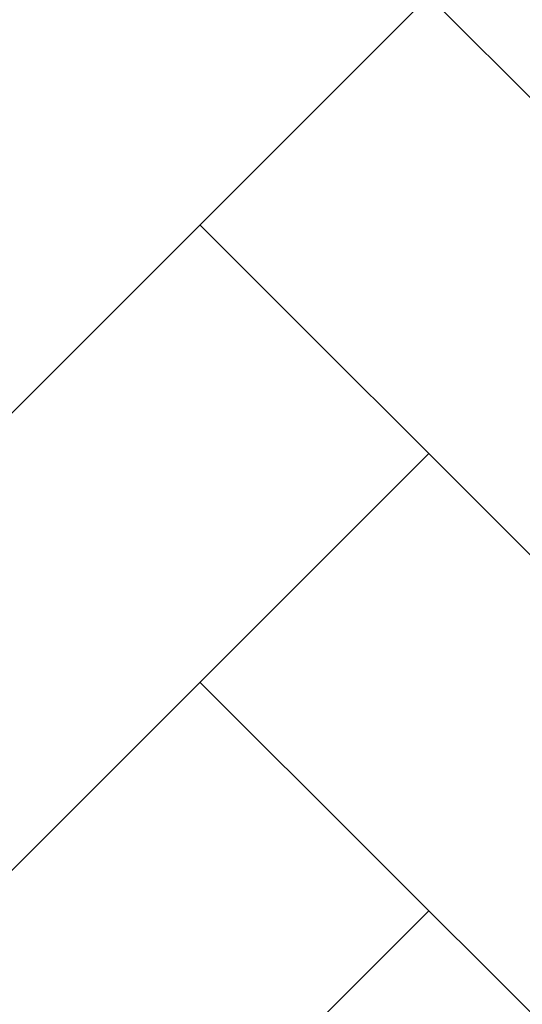
# Model space of a CAD drawing. Units: inches. Extents: x 3590 to 5167, y 65 to 1917.
# Tile 44 of 100: x 5003 to 5035, y 1388 to 1450. Entities that reach past the tile are written whole.
import ezdxf

# ---------------------------------------------------------------- set-up
doc = ezdxf.new("R2010")
doc.units = ezdxf.units.IN
doc.layers.add('A-FLOR-PATT', color=8, linetype='Continuous', lineweight=13)

msp = doc.modelspace()

# ---------------------------------------------------------------- hatches: boundary and pattern name
at = {"layer": 'A-FLOR-PATT', "transparency": 33554687}
h = msp.add_hatch(dxfattribs=at)
h.set_pattern_fill('AR-HBONE', color=256, scale=0.2)
h.set_pattern_definition([(45, (-588.972, 0), (0, 28.73682), [60.96, -20.32]), (135, (-574.604, 14.368), (3e-15, 28.73682), [60.96, -20.32])])
h.paths.add_polyline_path([(5071.274, 1796.999), (4933.274, 1796.999), (4933.274, 1753.999), (4962.774, 1753.999, -0.414214), (4928.774, 1719.999), (4933.274, 1718.999), (4933.274, 1334.999), (5071.274, 1334.999)])
h.paths.add_polyline_path([(4951.78, 1521.077), (4951.715, 1521.04), (4951.563, 1520.895)], flags=16)
h.paths.add_polyline_path([(4952.267, 1521.376), (4952.198, 1521.371), (4952.198, 1521.356)], flags=0)
h.paths.add_polyline_path([(4967.051, 1529.728), (4965.231, 1528.694), (4963.411, 1527.714), (4961.756, 1526.851), (4963.589, 1527.449), (4964.036, 1527.478), (4962.975, 1527.249), (4961.76, 1526.852), (4959.792, 1525.834), (4958.005, 1524.895), (4956.24, 1523.93), (4954.504, 1522.919), (4954.129, 1522.682), (4953.361, 1521.997), (4953.366, 1521.998), (4953.605, 1522.064), (4955.106, 1522.761), (4956.921, 1523.434), (4958.678, 1523.915), (4960.358, 1524.2), (4961.945, 1524.286), (4964.171, 1524.108), (4965.958, 1523.309), (4963.863, 1522.976), (4965.187, 1522.499), (4963.366, 1522.497), (4961.545, 1522.487), (4959.764, 1522.461), (4958.304, 1522.419), (4957.974, 1522.388), (4956.307, 1522.232), (4954.718, 1522.071), (4953.251, 1521.899), (4953.525, 1521.623), (4954.331, 1521.379), (4956.243, 1521.23), (4958.039, 1520.93), (4959.684, 1520.483), (4961.16, 1519.896), (4963.107, 1518.8), (4964.393, 1517.325), (4962.973, 1517.726), (4964.558, 1516.661), (4965.407, 1515.708), (4963.507, 1516.322), (4961.68, 1517.005), (4959.935, 1517.745), (4958.282, 1518.528), (4956.732, 1519.343), (4955.295, 1520.175), (4954.672, 1520.572), (4954.513, 1520.627), (4955.658, 1519.318), (4956.703, 1517.982), (4957.644, 1516.647), (4958.485, 1515.334), (4959.55, 1513.524), (4960.438, 1511.769), (4958.841, 1513.62), (4957.452, 1515.325), (4955.819, 1517.459), (4956.665, 1515.448), (4957.111, 1513.923), (4957.447, 1511.714), (4957.076, 1509.793), (4956.538, 1511.11), (4955.992, 1512.569), (4955.444, 1514.125), (4954.898, 1515.735), (4954.357, 1517.356), (4953.824, 1518.943), (4953.305, 1520.452), (4953.065, 1521.116), (4952.971, 1521.146), (4952.949, 1521.086), (4952.73, 1520.199), (4953.37, 1518.024), (4953.757, 1516.373), (4954.051, 1514.765), (4954.264, 1513.221), (4954.471, 1511.131), (4954.497, 1510.402), (4954.409, 1511.76), (4954.264, 1513.221), (4954.051, 1514.765), (4953.757, 1516.373), (4953.37, 1518.024), (4952.877, 1519.698), (4952.716, 1520.141), (4952.533, 1519.059), (4952.374, 1517.789), (4952.219, 1516.312), (4952.046, 1514.6), (4951.833, 1512.626), (4951.557, 1510.363), (4951.203, 1512.168), (4950.852, 1514.339), (4950.985, 1516.376), (4951.66, 1518.286), (4952.593, 1520.481), (4952.357, 1521.13), (4951.855, 1520.328), (4950.839, 1518.908), (4949.777, 1517.587), (4948.916, 1516.617), (4948.111, 1515.256), (4947.089, 1513.554), (4945.889, 1511.615), (4946.326, 1513.402), (4946.562, 1514.249), (4945.528, 1513.327), (4944.581, 1512.531), (4946.018, 1514.508), (4947.204, 1516.048), (4947.893, 1517.313), (4949.307, 1518.764), (4950.414, 1519.767), (4950.451, 1519.806), (4952.267, 1521.376), (4951.645, 1521.493), (4950.404, 1521.18), (4948.044, 1520.359), (4946.119, 1519.452), (4944.572, 1518.475), (4943.35, 1517.443), (4941.997, 1515.92), (4941.661, 1515.275), (4942.813, 1516.99), (4944.572, 1518.475), (4946.119, 1519.452), (4948.044, 1520.359), (4950.404, 1521.18), (4951.645, 1521.493), (4949.647, 1521.868), (4948.6, 1521.756), (4947.126, 1521.57), (4945.42, 1521.348), (4943.45, 1521.105), (4941.183, 1520.856), (4942.86, 1521.613), (4943.873, 1522.03), (4942.952, 1521.909), (4941.41, 1521.485), (4939.543, 1520.67), (4938.968, 1520.226), (4940.733, 1521.299), (4942.952, 1521.909), (4943.702, 1522.008), (4945.894, 1522.7), (4947.565, 1522.714), (4948.921, 1522.566), (4951.131, 1522.183), (4950.971, 1522.297), (4948.129, 1523.006), (4946.035, 1523.707), (4944.232, 1524.521), (4942.707, 1525.461), (4941.444, 1526.537), (4940.43, 1527.761), (4939.649, 1529.143), (4941.421, 1528.122), (4943.147, 1527.132), (4944.841, 1526.175), (4946.514, 1525.25), (4948.179, 1524.359), (4948.365, 1524.263), (4946.475, 1526.045), (4945.181, 1527.54), (4944.19, 1529.033), (4943.496, 1530.54), (4943.278, 1531.36), (4942.498, 1531.919), (4943.114, 1531.762), (4942.959, 1533.659), (4944.14, 1531.989), (4944.612, 1531.323), (4946.202, 1530.463), (4947.486, 1529.509), (4948.79, 1528.226), (4950.368, 1526.237), (4949.485, 1528.155), (4948.851, 1530.123), (4948.491, 1532.041), (4948.381, 1533.918), (4948.501, 1535.76), (4948.827, 1537.573), (4949.418, 1535.565), (4949.957, 1533.569), (4950.464, 1531.586), (4950.961, 1529.617), (4951.391, 1527.954), (4951.724, 1530.687), (4952.201, 1532.58), (4952.889, 1534.33), (4953.77, 1535.951), (4954.827, 1537.46), (4954.521, 1535.39), (4954.273, 1533.937), (4955.58, 1535.663), (4956.748, 1536.739), (4956.159, 1534.78), (4955.589, 1532.873), (4955.043, 1531.006), (4954.525, 1529.166), (4954.038, 1527.341), (4953.638, 1525.733), (4953.611, 1525.586), (4953.398, 1524.166), (4953.382, 1524.009), (4954.07, 1525.476), (4954.912, 1527.022), (4956.136, 1528.894), (4957.847, 1530.577), (4959.376, 1531.54), (4958.256, 1530.104), (4957.143, 1528.663), (4956.066, 1527.243), (4955.056, 1525.871), (4954.141, 1524.571), (4953.352, 1523.372), (4953.311, 1523.303), (4953.273, 1522.925), (4953.261, 1522.382), (4954.103, 1523.373), (4954.63, 1524.284), (4955.961, 1526.358), (4957.23, 1528.13), (4958.421, 1529.609), (4960.037, 1531.368), (4961.374, 1532.375), (4962.101, 1532.77), (4961.07, 1531.061), (4959.987, 1529.438), (4958.869, 1527.908), (4958.15, 1527.007), (4959.803, 1528.003), (4961.589, 1528.793), (4963.391, 1529.328), (4965.211, 1529.632)], flags=16)
h.paths.add_polyline_path([(4962.944, 1523.182), (4961.107, 1523.422), (4960.392, 1523.362), (4962.35, 1523.331)], flags=0)
h.paths.add_polyline_path([(5049.541, 1584.551), (5049.476, 1584.515), (5049.325, 1584.37)], flags=16)
h.paths.add_polyline_path([(5050.028, 1584.851), (5049.959, 1584.845), (5049.959, 1584.83)], flags=0)
h.paths.add_polyline_path([(5042.333, 1581.949), (5043.88, 1582.926), (5045.806, 1583.833), (5048.165, 1584.654), (5049.406, 1584.967), (5047.408, 1585.342), (5046.361, 1585.231), (5044.888, 1585.044), (5043.181, 1584.822), (5041.211, 1584.579), (5038.944, 1584.33), (5040.622, 1585.087), (5041.634, 1585.504), (5040.713, 1585.383), (5039.171, 1584.959), (5037.304, 1584.144), (5036.729, 1583.7), (5038.494, 1584.773), (5040.713, 1585.383), (5041.463, 1585.482), (5043.655, 1586.174), (5045.326, 1586.188), (5046.682, 1586.04), (5048.893, 1585.657), (5048.732, 1585.771), (5045.891, 1586.48), (5043.796, 1587.181), (5041.994, 1587.996), (5040.468, 1588.935), (5039.205, 1590.011), (5038.191, 1591.235), (5037.41, 1592.617), (5039.182, 1591.596), (5040.909, 1590.607), (5042.602, 1589.649), (5044.275, 1588.724), (5045.94, 1587.833), (5046.126, 1587.738), (5044.237, 1589.519), (5042.942, 1591.015), (5041.952, 1592.508), (5041.257, 1594.014), (5041.039, 1594.834), (5040.26, 1595.393), (5040.875, 1595.237), (5040.721, 1597.133), (5041.901, 1595.463), (5042.373, 1594.798), (5043.963, 1593.938), (5045.247, 1592.983), (5046.552, 1591.701), (5048.129, 1589.712), (5047.247, 1591.63), (5046.613, 1593.597), (5046.252, 1595.515), (5046.142, 1597.392), (5046.262, 1599.234), (5046.588, 1601.047), (5047.179, 1599.039), (5047.718, 1597.043), (5048.225, 1595.06), (5048.722, 1593.091), (5049.152, 1591.429), (5049.485, 1594.161), (5049.962, 1596.054), (5050.65, 1597.804), (5051.532, 1599.425), (5052.589, 1600.934), (5052.283, 1598.864), (5052.034, 1597.411), (5053.341, 1599.137), (5054.509, 1600.213), (5053.92, 1598.254), (5053.35, 1596.348), (5052.805, 1594.48), (5052.286, 1592.64), (5051.799, 1590.815), (5051.4, 1589.207), (5051.373, 1589.06), (5051.159, 1587.64), (5051.143, 1587.483), (5051.831, 1588.95), (5052.673, 1590.496), (5053.898, 1592.368), (5055.608, 1594.051), (5057.137, 1595.014), (5056.017, 1593.578), (5054.904, 1592.137), (5053.828, 1590.717), (5052.817, 1589.345), (5051.902, 1588.046), (5051.113, 1586.846), (5051.072, 1586.777), (5051.034, 1586.399), (5051.022, 1585.856), (5051.864, 1586.847), (5052.391, 1587.758), (5053.723, 1589.832), (5054.991, 1591.604), (5056.182, 1593.083), (5057.798, 1594.842), (5059.135, 1595.849), (5059.863, 1596.244), (5058.831, 1594.535), (5057.749, 1592.912), (5056.63, 1591.382), (5055.912, 1590.482), (5057.564, 1591.477), (5059.35, 1592.267), (5061.152, 1592.802), (5062.972, 1593.106), (5064.812, 1593.203), (5062.992, 1592.169), (5061.172, 1591.188), (5059.518, 1590.325), (5061.35, 1590.924), (5061.797, 1590.952), (5060.737, 1590.723), (5059.521, 1590.326), (5057.553, 1589.308), (5055.766, 1588.369), (5054.002, 1587.404), (5052.265, 1586.393), (5051.891, 1586.156), (5051.122, 1585.471), (5051.127, 1585.472), (5051.366, 1585.538), (5052.867, 1586.235), (5054.682, 1586.908), (5056.439, 1587.389), (5058.12, 1587.675), (5059.706, 1587.76), (5061.933, 1587.583), (5063.719, 1586.783), (5061.624, 1586.45), (5062.949, 1585.973), (5061.127, 1585.971), (5059.307, 1585.961), (5057.525, 1585.935), (5056.065, 1585.893), (5055.735, 1585.862), (5054.068, 1585.707), (5052.479, 1585.546), (5051.012, 1585.373), (5051.286, 1585.097), (5052.092, 1584.853), (5054.004, 1584.704), (5055.8, 1584.404), (5057.446, 1583.958), (5058.921, 1583.37), (5060.868, 1582.274), (5062.154, 1580.799), (5060.734, 1581.2), (5062.32, 1580.135), (5063.168, 1579.182), (5061.269, 1579.796), (5059.441, 1580.479), (5057.696, 1581.219), (5056.043, 1582.003), (5054.493, 1582.817), (5053.057, 1583.649), (5052.433, 1584.047), (5052.274, 1584.101), (5053.42, 1582.793), (5054.464, 1581.457), (5055.405, 1580.121), (5056.247, 1578.809), (5057.311, 1576.998), (5058.199, 1575.244), (5056.602, 1577.094), (5055.213, 1578.799), (5053.58, 1580.933), (5054.427, 1578.922), (5054.872, 1577.397), (5055.208, 1575.189), (5054.838, 1573.267), (5054.299, 1574.584), (5053.754, 1576.043), (5053.206, 1577.599), (5052.659, 1579.209), (5052.118, 1580.83), (5051.585, 1582.417), (5051.066, 1583.927), (5050.826, 1584.59), (5050.733, 1584.62), (5050.711, 1584.561), (5050.491, 1583.673), (5051.131, 1581.498), (5051.518, 1579.847), (5051.813, 1578.24), (5052.026, 1576.695), (5052.233, 1574.605), (5052.258, 1573.876), (5052.17, 1575.234), (5052.026, 1576.695), (5051.813, 1578.24), (5051.518, 1579.847), (5051.131, 1581.498), (5050.638, 1583.172), (5050.477, 1583.615), (5050.294, 1582.533), (5050.136, 1581.263), (5049.981, 1579.786), (5049.807, 1578.074), (5049.594, 1576.1), (5049.318, 1573.837), (5048.965, 1575.642), (5048.613, 1577.813), (5048.747, 1579.85), (5049.421, 1581.76), (5050.354, 1583.955), (5050.118, 1584.604), (5049.616, 1583.802), (5048.6, 1582.382), (5047.538, 1581.061), (5046.677, 1580.091), (5045.872, 1578.73), (5044.85, 1577.028), (5043.651, 1575.089), (5044.087, 1576.877), (5044.324, 1577.723), (5043.289, 1576.801), (5042.342, 1576.005), (5043.779, 1577.982), (5044.966, 1579.522), (5045.655, 1580.787), (5047.068, 1582.239), (5048.175, 1583.241), (5048.213, 1583.28), (5050.028, 1584.851), (5049.406, 1584.967), (5048.165, 1584.654), (5045.806, 1583.833), (5043.88, 1582.926), (5042.333, 1581.949), (5041.111, 1580.917), (5039.758, 1579.394), (5039.423, 1578.749), (5040.575, 1580.464)], flags=16)
h.paths.add_polyline_path([(4954.799, 1533.12), (4954.262, 1532.079), (4953.831, 1530.935), (4953.505, 1529.636), (4953.283, 1528.133), (4953.167, 1526.376), (4953.156, 1524.315), (4953.277, 1521.236), (4952.802, 1521.842), (4951.557, 1521.998), (4950.976, 1521.961), (4952.661, 1521.941), (4952.802, 1521.842), (4953.152, 1523.593), (4953.167, 1526.376), (4953.283, 1528.133), (4953.609, 1530.346), (4954.456, 1532.592)], flags=0)
h.paths.add_polyline_path([(5050.563, 1585.316), (5049.318, 1585.472), (5048.737, 1585.435), (5050.422, 1585.415), (5050.563, 1585.316), (5050.914, 1587.067), (5050.928, 1589.851), (5051.045, 1591.607), (5051.371, 1593.82), (5052.217, 1596.066), (5052.56, 1596.594), (5052.024, 1595.554), (5051.592, 1594.409), (5051.266, 1593.11), (5051.045, 1591.607), (5050.928, 1589.851), (5050.918, 1587.789), (5051.038, 1584.71)], flags=0)
h.paths.add_polyline_path([(5058.153, 1586.836), (5060.111, 1586.805), (5060.705, 1586.656), (5058.868, 1586.896)], flags=0)
h.paths.add_polyline_path([(5049.541, 1430.936), (5049.476, 1430.9), (5049.325, 1430.755)], flags=16)
h.paths.add_polyline_path([(5050.028, 1431.236), (5049.959, 1431.231), (5049.959, 1431.215)], flags=0)
h.paths.add_polyline_path([(5046.588, 1447.432), (5047.179, 1445.425), (5047.718, 1443.429), (5048.225, 1441.446), (5048.722, 1439.476), (5049.152, 1437.814), (5049.485, 1440.546), (5049.962, 1442.439), (5050.65, 1444.189), (5051.532, 1445.811), (5052.589, 1447.319), (5052.283, 1445.249), (5052.034, 1443.796), (5053.341, 1445.522), (5054.509, 1446.598), (5053.92, 1444.64), (5053.35, 1442.733), (5052.805, 1440.865), (5052.286, 1439.025), (5051.799, 1437.201), (5051.4, 1435.592), (5051.373, 1435.445), (5051.159, 1434.025), (5051.143, 1433.868), (5051.831, 1435.335), (5052.673, 1436.881), (5053.898, 1438.753), (5055.608, 1440.436), (5057.137, 1441.4), (5056.017, 1439.963), (5054.904, 1438.522), (5053.828, 1437.102), (5052.817, 1435.73), (5051.902, 1434.431), (5051.113, 1433.231), (5051.072, 1433.162), (5051.034, 1432.784), (5051.022, 1432.242), (5051.864, 1433.232), (5052.391, 1434.143), (5053.723, 1436.217), (5054.991, 1437.989), (5056.182, 1439.468), (5057.798, 1441.227), (5059.135, 1442.235), (5059.863, 1442.629), (5058.831, 1440.921), (5057.749, 1439.298), (5056.63, 1437.767), (5055.912, 1436.867), (5057.564, 1437.863), (5059.35, 1438.652), (5061.152, 1439.187), (5062.972, 1439.491), (5064.812, 1439.588), (5062.992, 1438.554), (5061.172, 1437.573), (5059.518, 1436.71), (5061.35, 1437.309), (5061.797, 1437.337), (5060.737, 1437.108), (5059.521, 1436.711), (5057.553, 1435.693), (5055.766, 1434.754), (5054.002, 1433.789), (5052.265, 1432.778), (5051.891, 1432.541), (5051.122, 1431.856), (5051.127, 1431.857), (5051.366, 1431.923), (5052.867, 1432.62), (5054.682, 1433.293), (5056.439, 1433.775), (5058.12, 1434.06), (5059.706, 1434.145), (5061.933, 1433.968), (5063.719, 1433.168), (5061.624, 1432.835), (5062.949, 1432.358), (5061.127, 1432.357), (5059.307, 1432.346), (5057.525, 1432.32), (5056.065, 1432.278), (5055.735, 1432.248), (5054.068, 1432.092), (5052.479, 1431.931), (5051.012, 1431.759), (5051.286, 1431.482), (5052.092, 1431.238), (5054.004, 1431.089), (5055.8, 1430.789), (5057.446, 1430.343), (5058.921, 1429.755), (5060.868, 1428.66), (5062.154, 1427.185), (5060.734, 1427.585), (5062.32, 1426.52), (5063.168, 1425.567), (5061.269, 1426.181), (5059.441, 1426.865), (5057.696, 1427.604), (5056.043, 1428.388), (5054.493, 1429.202), (5053.057, 1430.034), (5052.433, 1430.432), (5052.274, 1430.487), (5053.42, 1429.178), (5054.464, 1427.842), (5055.405, 1426.506), (5056.247, 1425.194), (5057.311, 1423.383), (5058.199, 1421.629), (5056.602, 1423.479), (5055.213, 1425.184), (5053.58, 1427.318), (5054.427, 1425.307), (5054.872, 1423.782), (5055.208, 1421.574), (5054.838, 1419.652), (5054.299, 1420.97), (5053.754, 1422.428), (5053.206, 1423.984), (5052.659, 1425.595), (5052.118, 1427.215), (5051.585, 1428.802), (5051.066, 1430.312), (5050.826, 1430.975), (5050.733, 1431.005), (5050.711, 1430.946), (5050.491, 1430.058), (5051.131, 1427.883), (5051.518, 1426.232), (5051.813, 1424.625), (5052.026, 1423.081), (5052.233, 1420.991), (5052.258, 1420.261), (5052.17, 1421.619), (5052.026, 1423.081), (5051.813, 1424.625), (5051.518, 1426.232), (5051.131, 1427.883), (5050.638, 1429.558), (5050.477, 1430.001), (5050.294, 1428.918), (5050.136, 1427.648), (5049.981, 1426.171), (5049.807, 1424.459), (5049.594, 1422.485), (5049.318, 1420.222), (5048.965, 1422.028), (5048.613, 1424.199), (5048.747, 1426.235), (5049.421, 1428.146), (5050.354, 1430.34), (5050.118, 1430.989), (5049.616, 1430.187), (5048.6, 1428.768), (5047.538, 1427.446), (5046.677, 1426.477), (5045.872, 1425.116), (5044.85, 1423.413), (5043.651, 1421.474), (5044.087, 1423.262), (5044.324, 1424.109), (5043.289, 1423.186), (5042.342, 1422.391), (5043.779, 1424.368), (5044.966, 1425.907), (5045.655, 1427.173), (5047.068, 1428.624), (5048.175, 1429.627), (5048.213, 1429.666), (5050.028, 1431.236), (5049.406, 1431.353), (5048.165, 1431.039), (5045.806, 1430.218), (5043.88, 1429.311), (5042.333, 1428.334), (5041.111, 1427.302), (5039.758, 1425.779), (5039.423, 1425.134), (5040.575, 1426.849), (5042.333, 1428.334), (5043.88, 1429.311), (5045.806, 1430.218), (5048.165, 1431.039), (5049.406, 1431.353), (5047.408, 1431.727), (5046.361, 1431.616), (5044.888, 1431.429), (5043.181, 1431.207), (5041.211, 1430.964), (5038.944, 1430.715), (5040.622, 1431.472), (5041.634, 1431.89), (5040.713, 1431.769), (5039.171, 1431.345), (5037.304, 1430.53), (5036.729, 1430.085), (5038.494, 1431.158), (5040.713, 1431.769), (5041.463, 1431.867), (5043.655, 1432.559), (5045.326, 1432.573), (5046.682, 1432.425), (5048.893, 1432.042), (5048.732, 1432.156), (5045.891, 1432.865), (5043.796, 1433.566), (5041.994, 1434.381), (5040.468, 1435.321), (5039.205, 1436.396), (5038.191, 1437.62), (5037.41, 1439.002), (5039.182, 1437.982), (5040.909, 1436.992), (5042.602, 1436.034), (5044.275, 1435.109), (5045.94, 1434.218), (5046.126, 1434.123), (5044.237, 1435.904), (5042.942, 1437.4), (5041.952, 1438.893), (5041.257, 1440.399), (5041.039, 1441.219), (5040.26, 1441.778), (5040.875, 1441.622), (5040.721, 1443.518), (5041.901, 1441.848), (5042.373, 1441.183), (5043.963, 1440.323), (5045.247, 1439.369), (5046.552, 1438.086), (5048.129, 1436.097), (5047.247, 1438.015), (5046.613, 1439.982), (5046.252, 1441.901), (5046.142, 1443.778), (5046.262, 1445.619)], flags=16)
h.paths.add_polyline_path([(5052.382, 1444.255), (5051.623, 1442.78), (5052.024, 1441.939), (5052.56, 1442.98)], flags=0)
h.paths.add_polyline_path([(5050.563, 1431.701), (5049.318, 1431.857), (5048.737, 1431.821), (5050.422, 1431.8)], flags=0)
h.paths.add_polyline_path([(5058.153, 1433.221), (5060.111, 1433.19), (5060.705, 1433.041), (5058.868, 1433.281)], flags=0)
h.paths.add_polyline_path([(5049.541, 1352.285), (5049.476, 1352.249), (5049.325, 1352.104)], flags=16)
h.paths.add_polyline_path([(5050.028, 1352.585), (5049.959, 1352.58), (5049.959, 1352.564)], flags=0)
h.paths.add_polyline_path([(5046.588, 1368.781), (5047.179, 1366.774), (5047.718, 1364.778), (5048.225, 1362.795), (5048.722, 1360.825), (5049.152, 1359.163), (5049.485, 1361.896), (5049.962, 1363.789), (5050.65, 1365.538), (5051.532, 1367.16), (5052.589, 1368.669), (5052.283, 1366.598), (5052.034, 1365.145), (5053.341, 1366.871), (5054.509, 1367.947), (5053.92, 1365.989), (5053.35, 1364.082), (5052.805, 1362.214), (5052.286, 1360.374), (5051.799, 1358.55), (5051.4, 1356.942), (5051.373, 1356.794), (5051.159, 1355.374), (5051.143, 1355.218), (5051.831, 1356.684), (5052.673, 1358.23), (5053.898, 1360.102), (5055.608, 1361.786), (5057.137, 1362.749), (5056.017, 1361.313), (5054.904, 1359.872), (5053.828, 1358.452), (5052.817, 1357.079), (5051.902, 1355.78), (5051.113, 1354.581), (5051.072, 1354.512), (5051.034, 1354.133), (5051.022, 1353.591), (5051.864, 1354.581), (5052.391, 1355.492), (5053.723, 1357.566), (5054.991, 1359.338), (5056.182, 1360.817), (5057.798, 1362.577), (5059.135, 1363.584), (5059.863, 1363.979), (5058.831, 1362.27), (5057.749, 1360.647), (5056.63, 1359.117), (5055.912, 1358.216), (5057.564, 1359.212), (5059.35, 1360.001), (5061.152, 1360.536), (5062.972, 1360.841), (5064.812, 1360.937), (5062.992, 1359.903), (5061.172, 1358.923), (5059.518, 1358.059), (5061.35, 1358.658), (5061.797, 1358.687), (5060.737, 1358.458), (5059.521, 1358.061), (5057.553, 1357.043), (5055.766, 1356.103), (5054.002, 1355.138), (5052.265, 1354.127), (5051.891, 1353.89), (5051.122, 1353.206), (5051.127, 1353.206), (5051.366, 1353.272), (5052.867, 1353.969), (5054.682, 1354.643), (5056.439, 1355.124), (5058.12, 1355.409), (5059.706, 1355.495), (5061.933, 1355.317), (5063.719, 1354.518), (5061.624, 1354.184), (5062.949, 1353.708), (5061.127, 1353.706), (5059.307, 1353.695), (5057.525, 1353.669), (5056.065, 1353.627), (5055.735, 1353.597), (5054.068, 1353.441), (5052.479, 1353.28), (5051.012, 1353.108), (5051.286, 1352.831), (5052.092, 1352.587), (5054.004, 1352.439), (5055.8, 1352.138), (5057.446, 1351.692), (5058.921, 1351.104), (5060.868, 1350.009), (5062.154, 1348.534), (5060.734, 1348.935), (5062.32, 1347.869), (5063.168, 1346.916), (5061.269, 1347.53), (5059.441, 1348.214), (5057.696, 1348.954), (5056.043, 1349.737), (5054.493, 1350.551), (5053.057, 1351.383), (5052.433, 1351.781), (5052.274, 1351.836), (5053.42, 1350.527), (5054.464, 1349.191), (5055.405, 1347.855), (5056.247, 1346.543), (5057.311, 1344.733), (5058.199, 1342.978), (5056.602, 1344.828), (5055.213, 1346.534), (5053.58, 1348.667), (5054.427, 1346.656), (5054.872, 1345.132), (5055.208, 1342.923), (5054.838, 1341.002), (5054.299, 1342.319), (5053.754, 1343.778), (5053.206, 1345.334), (5052.659, 1346.944), (5052.118, 1348.564), (5051.585, 1350.151), (5051.066, 1351.661), (5050.826, 1352.324), (5050.733, 1352.355), (5050.711, 1352.295), (5050.491, 1351.408), (5051.131, 1349.232), (5051.518, 1347.581), (5051.813, 1345.974), (5052.026, 1344.43), (5052.233, 1342.34), (5052.258, 1341.61), (5052.17, 1342.969), (5052.026, 1344.43), (5051.813, 1345.974), (5051.518, 1347.581), (5051.131, 1349.232), (5050.638, 1350.907), (5050.477, 1351.35), (5050.294, 1350.267), (5050.136, 1348.997), (5049.981, 1347.52), (5049.807, 1345.809), (5049.594, 1343.835), (5049.318, 1341.571), (5048.965, 1343.377), (5048.613, 1345.548), (5048.747, 1347.585), (5049.421, 1349.495), (5050.354, 1351.689), (5050.118, 1352.339), (5049.616, 1351.536), (5048.6, 1350.117), (5047.538, 1348.795), (5046.677, 1347.826), (5045.872, 1346.465), (5044.85, 1344.763), (5043.651, 1342.824), (5044.087, 1344.611), (5044.324, 1345.458), (5043.289, 1344.535), (5042.342, 1343.74), (5043.779, 1345.717), (5044.966, 1347.256), (5045.655, 1348.522), (5047.068, 1349.973), (5048.175, 1350.976), (5048.213, 1351.015), (5050.028, 1352.585), (5049.406, 1352.702), (5048.165, 1352.388), (5045.806, 1351.567), (5043.88, 1350.661), (5042.333, 1349.683), (5041.111, 1348.651), (5039.758, 1347.128), (5039.423, 1346.483), (5040.575, 1348.198), (5042.333, 1349.683), (5043.88, 1350.661), (5045.806, 1351.567), (5048.165, 1352.388), (5049.406, 1352.702), (5047.408, 1353.076), (5046.361, 1352.965), (5044.888, 1352.779), (5043.181, 1352.556), (5041.211, 1352.313), (5038.944, 1352.065), (5040.622, 1352.821), (5041.634, 1353.239), (5040.713, 1353.118), (5039.171, 1352.694), (5037.304, 1351.879), (5036.729, 1351.434), (5038.494, 1352.508), (5040.713, 1353.118), (5041.463, 1353.216), (5043.655, 1353.909), (5045.326, 1353.923), (5046.682, 1353.774), (5048.893, 1353.391), (5048.732, 1353.506), (5045.891, 1354.214), (5043.796, 1354.915), (5041.994, 1355.73), (5040.468, 1356.67), (5039.205, 1357.746), (5038.191, 1358.969), (5037.41, 1360.352), (5039.182, 1359.331), (5040.909, 1358.341), (5042.602, 1357.383), (5044.275, 1356.458), (5045.94, 1355.567), (5046.126, 1355.472), (5044.237, 1357.253), (5042.942, 1358.749), (5041.952, 1360.242), (5041.257, 1361.748), (5041.039, 1362.568), (5040.26, 1363.128), (5040.875, 1362.971), (5040.721, 1364.867), (5041.901, 1363.197), (5042.373, 1362.532), (5043.963, 1361.672), (5045.247, 1360.718), (5046.552, 1359.435), (5048.129, 1357.446), (5047.247, 1359.364), (5046.613, 1361.331), (5046.252, 1363.25), (5046.142, 1365.127), (5046.262, 1366.969)], flags=16)
h.paths.add_polyline_path([(5052.382, 1365.604), (5051.623, 1364.129), (5052.024, 1363.288), (5052.56, 1364.329)], flags=0)
h.paths.add_polyline_path([(4951.78, 1698.041), (4951.715, 1698.005), (4951.563, 1697.859)], flags=16)
h.paths.add_polyline_path([(4952.267, 1698.341), (4952.198, 1698.335), (4952.198, 1698.32)], flags=0)
h.paths.add_polyline_path([(4957.076, 1686.757), (4956.538, 1688.074), (4955.992, 1689.533), (4955.444, 1691.089), (4954.898, 1692.699), (4954.357, 1694.32), (4953.824, 1695.907), (4953.305, 1697.417), (4953.065, 1698.08), (4952.971, 1698.11), (4952.949, 1698.051), (4952.73, 1697.163), (4953.37, 1694.988), (4953.757, 1693.337), (4954.051, 1691.729), (4954.264, 1690.185), (4954.471, 1688.095), (4954.497, 1687.366), (4954.409, 1688.724), (4954.264, 1690.185), (4954.051, 1691.729), (4953.757, 1693.337), (4953.37, 1694.988), (4952.877, 1696.662), (4952.716, 1697.105), (4952.533, 1696.023), (4952.374, 1694.753), (4952.219, 1693.276), (4952.046, 1691.564), (4951.833, 1689.59), (4951.557, 1687.327), (4951.203, 1689.132), (4950.852, 1691.303), (4950.985, 1693.34), (4951.66, 1695.25), (4952.593, 1697.445), (4952.357, 1698.094), (4951.855, 1697.292), (4950.839, 1695.872), (4949.777, 1694.551), (4948.916, 1693.581), (4948.111, 1692.22), (4947.089, 1690.518), (4945.889, 1688.579), (4946.326, 1690.366), (4946.562, 1691.213), (4945.528, 1690.291), (4944.581, 1689.495), (4946.018, 1691.472), (4947.204, 1693.012), (4947.893, 1694.277), (4949.307, 1695.729), (4950.414, 1696.731), (4950.451, 1696.77), (4952.267, 1698.341), (4951.645, 1698.457), (4950.404, 1698.144), (4948.044, 1697.323), (4946.119, 1696.416), (4944.572, 1695.439), (4943.35, 1694.407), (4941.997, 1692.884), (4941.661, 1692.239), (4942.813, 1693.954), (4944.572, 1695.439), (4946.119, 1696.416), (4948.044, 1697.323), (4950.404, 1698.144), (4951.645, 1698.457), (4949.647, 1698.832), (4948.6, 1698.72), (4947.126, 1698.534), (4945.42, 1698.312), (4943.45, 1698.069), (4941.183, 1697.82), (4942.86, 1698.577), (4943.873, 1698.994), (4942.952, 1698.873), (4941.41, 1698.449), (4939.543, 1697.634), (4938.968, 1697.19), (4940.733, 1698.263), (4942.952, 1698.873), (4943.702, 1698.972), (4945.894, 1699.664), (4947.565, 1699.678), (4948.921, 1699.53), (4951.131, 1699.147), (4950.971, 1699.261), (4948.129, 1699.97), (4946.035, 1700.671), (4944.232, 1701.486), (4942.707, 1702.425), (4941.444, 1703.501), (4940.43, 1704.725), (4939.649, 1706.107), (4941.421, 1705.086), (4943.147, 1704.097), (4944.841, 1703.139), (4946.514, 1702.214), (4948.179, 1701.323), (4948.365, 1701.227), (4946.475, 1703.009), (4945.181, 1704.505), (4944.19, 1705.997), (4943.496, 1707.504), (4943.278, 1708.324), (4942.498, 1708.883), (4943.114, 1708.727), (4942.959, 1710.623), (4944.14, 1708.953), (4944.612, 1708.287), (4946.202, 1707.428), (4947.486, 1706.473), (4948.79, 1705.191), (4950.368, 1703.202), (4949.485, 1705.12), (4948.851, 1707.087), (4948.491, 1709.005), (4948.381, 1710.882), (4948.501, 1712.724), (4948.827, 1714.537), (4949.418, 1712.529), (4949.957, 1710.533), (4950.464, 1708.55), (4950.961, 1706.581), (4951.391, 1704.919), (4951.724, 1707.651), (4952.201, 1709.544), (4952.889, 1711.294), (4953.77, 1712.915), (4954.827, 1714.424), (4954.521, 1712.354), (4954.273, 1710.901), (4955.58, 1712.627), (4956.748, 1713.703), (4956.159, 1711.744), (4955.589, 1709.837), (4955.043, 1707.97), (4954.525, 1706.13), (4954.038, 1704.305), (4953.638, 1702.697), (4953.611, 1702.55), (4953.398, 1701.13), (4953.382, 1700.973), (4954.07, 1702.44), (4954.912, 1703.986), (4956.136, 1705.858), (4957.847, 1707.541), (4959.376, 1708.504), (4958.256, 1707.068), (4957.143, 1705.627), (4956.066, 1704.207), (4955.056, 1702.835), (4954.141, 1701.536), (4953.352, 1700.336), (4953.311, 1700.267), (4953.273, 1699.889), (4953.261, 1699.346), (4954.103, 1700.337), (4954.63, 1701.248), (4955.961, 1703.322), (4957.23, 1705.094), (4958.421, 1706.573), (4960.037, 1708.332), (4961.374, 1709.339), (4962.101, 1709.734), (4961.07, 1708.025), (4959.987, 1706.402), (4958.869, 1704.872), (4958.15, 1703.972), (4959.803, 1704.967), (4961.589, 1705.757), (4963.391, 1706.292), (4965.211, 1706.596), (4967.051, 1706.692), (4965.231, 1705.659), (4963.411, 1704.678), (4961.756, 1703.815), (4963.589, 1704.413), (4964.036, 1704.442), (4962.975, 1704.213), (4961.76, 1703.816), (4959.792, 1702.798), (4958.005, 1701.859), (4956.24, 1700.894), (4954.504, 1699.883), (4954.129, 1699.646), (4953.361, 1698.961), (4953.366, 1698.962), (4953.605, 1699.028), (4955.106, 1699.725), (4956.921, 1700.398), (4958.678, 1700.879), (4960.358, 1701.164), (4961.945, 1701.25), (4964.171, 1701.073), (4965.958, 1700.273), (4963.863, 1699.94), (4965.187, 1699.463), (4963.366, 1699.461), (4961.545, 1699.451), (4959.764, 1699.425), (4958.304, 1699.383), (4957.974, 1699.352), (4956.307, 1699.197), (4954.718, 1699.036), (4953.251, 1698.863), (4953.525, 1698.587), (4954.331, 1698.343), (4956.243, 1698.194), (4958.039, 1697.894), (4959.684, 1697.447), (4961.16, 1696.86), (4963.107, 1695.764), (4964.393, 1694.289), (4962.973, 1694.69), (4964.558, 1693.625), (4965.407, 1692.672), (4963.507, 1693.286), (4961.68, 1693.969), (4959.935, 1694.709), (4958.282, 1695.492), (4956.732, 1696.307), (4955.295, 1697.139), (4954.672, 1697.536), (4954.513, 1697.591), (4955.658, 1696.282), (4956.703, 1694.946), (4957.644, 1693.611), (4958.485, 1692.298), (4959.55, 1690.488), (4960.438, 1688.733), (4958.841, 1690.584), (4957.452, 1692.289), (4955.819, 1694.423), (4956.665, 1692.412), (4957.111, 1690.887), (4957.447, 1688.678)], flags=16)
h.paths.add_polyline_path([(5050.563, 1353.05), (5049.318, 1353.207), (5048.737, 1353.17), (5050.422, 1353.15)], flags=0)
h.paths.add_polyline_path([(4951.78, 1351.486), (4951.715, 1351.45), (4951.563, 1351.305)], flags=16)
h.paths.add_polyline_path([(4952.267, 1351.786), (4952.198, 1351.78), (4952.198, 1351.765)], flags=0)
h.paths.add_polyline_path([(4954.827, 1367.869), (4954.521, 1365.799), (4954.273, 1364.346), (4955.58, 1366.072), (4956.748, 1367.148), (4956.159, 1365.19), (4955.589, 1363.283), (4955.043, 1361.415), (4954.525, 1359.575), (4954.038, 1357.751), (4953.638, 1356.142), (4953.611, 1355.995), (4953.398, 1354.575), (4953.382, 1354.418), (4954.07, 1355.885), (4954.912, 1357.431), (4956.136, 1359.303), (4957.847, 1360.986), (4959.376, 1361.95), (4958.256, 1360.513), (4957.143, 1359.072), (4956.066, 1357.652), (4955.056, 1356.28), (4954.141, 1354.981), (4953.352, 1353.781), (4953.311, 1353.712), (4953.273, 1353.334), (4953.261, 1352.792), (4954.103, 1353.782), (4954.63, 1354.693), (4955.961, 1356.767), (4957.23, 1358.539), (4958.421, 1360.018), (4960.037, 1361.777), (4961.374, 1362.785), (4962.101, 1363.179), (4961.07, 1361.471), (4959.987, 1359.848), (4958.869, 1358.317), (4958.15, 1357.417), (4959.803, 1358.413), (4961.589, 1359.202), (4963.391, 1359.737), (4965.211, 1360.041), (4967.051, 1360.138), (4965.231, 1359.104), (4963.411, 1358.123), (4961.756, 1357.26), (4963.589, 1357.859), (4964.036, 1357.887), (4962.975, 1357.658), (4961.76, 1357.261), (4959.792, 1356.243), (4958.005, 1355.304), (4956.24, 1354.339), (4954.504, 1353.328), (4954.129, 1353.091), (4953.361, 1352.406), (4953.366, 1352.407), (4953.605, 1352.473), (4955.106, 1353.17), (4956.921, 1353.843), (4958.678, 1354.325), (4960.358, 1354.61), (4961.945, 1354.695), (4964.171, 1354.518), (4965.958, 1353.718), (4963.863, 1353.385), (4965.187, 1352.908), (4963.366, 1352.907), (4961.545, 1352.896), (4959.764, 1352.87), (4958.304, 1352.828), (4957.974, 1352.798), (4956.307, 1352.642), (4954.718, 1352.481), (4953.251, 1352.309), (4953.525, 1352.032), (4954.331, 1351.788), (4956.243, 1351.639), (4958.039, 1351.339), (4959.684, 1350.893), (4961.16, 1350.305), (4963.107, 1349.21), (4964.393, 1347.735), (4962.973, 1348.135), (4964.558, 1347.07), (4965.407, 1346.117), (4963.507, 1346.731), (4961.68, 1347.414), (4959.935, 1348.154), (4958.282, 1348.938), (4956.732, 1349.752), (4955.295, 1350.584), (4954.672, 1350.982), (4954.513, 1351.036), (4955.658, 1349.728), (4956.703, 1348.392), (4957.644, 1347.056), (4958.485, 1345.744), (4959.55, 1343.933), (4960.438, 1342.179), (4958.841, 1344.029), (4957.452, 1345.734), (4955.819, 1347.868), (4956.665, 1345.857), (4957.111, 1344.332), (4957.447, 1342.124), (4957.076, 1340.202), (4956.538, 1341.52), (4955.992, 1342.978), (4955.444, 1344.534), (4954.898, 1346.145), (4954.357, 1347.765), (4953.824, 1349.352), (4953.305, 1350.862), (4953.065, 1351.525), (4952.971, 1351.555), (4952.949, 1351.496), (4952.73, 1350.608), (4953.37, 1348.433), (4953.757, 1346.782), (4954.051, 1345.175), (4954.264, 1343.631), (4954.471, 1341.541), (4954.497, 1340.811), (4954.409, 1342.169), (4954.264, 1343.631), (4954.051, 1345.175), (4953.757, 1346.782), (4953.37, 1348.433), (4952.877, 1350.108), (4952.716, 1350.551), (4952.533, 1349.468), (4952.374, 1348.198), (4952.219, 1346.721), (4952.046, 1345.009), (4951.833, 1343.035), (4951.557, 1340.772), (4951.203, 1342.578), (4950.852, 1344.749), (4950.985, 1346.785), (4951.66, 1348.696), (4952.593, 1350.89), (4952.357, 1351.539), (4951.855, 1350.737), (4950.839, 1349.318), (4949.777, 1347.996), (4948.916, 1347.027), (4948.111, 1345.665), (4947.089, 1343.963), (4945.889, 1342.024), (4946.326, 1343.812), (4946.562, 1344.659), (4945.528, 1343.736), (4944.581, 1342.941), (4946.018, 1344.918), (4947.204, 1346.457), (4947.893, 1347.723), (4949.307, 1349.174), (4950.414, 1350.177), (4950.451, 1350.216), (4952.267, 1351.786), (4951.645, 1351.903), (4950.404, 1351.589), (4948.044, 1350.768), (4946.119, 1349.861), (4944.572, 1348.884), (4943.35, 1347.852), (4941.997, 1346.329), (4941.661, 1345.684), (4942.813, 1347.399), (4944.572, 1348.884), (4946.119, 1349.861), (4948.044, 1350.768), (4950.404, 1351.589), (4951.645, 1351.903), (4949.647, 1352.277), (4948.6, 1352.166), (4947.126, 1351.979), (4945.42, 1351.757), (4943.45, 1351.514), (4941.183, 1351.265), (4942.86, 1352.022), (4943.873, 1352.44), (4942.952, 1352.319), (4941.41, 1351.895), (4939.543, 1351.08), (4938.968, 1350.635), (4940.733, 1351.708), (4942.952, 1352.319), (4943.702, 1352.417), (4945.894, 1353.109), (4947.565, 1353.123), (4948.921, 1352.975), (4951.131, 1352.592), (4950.971, 1352.706), (4948.129, 1353.415), (4946.035, 1354.116), (4944.232, 1354.931), (4942.707, 1355.871), (4941.444, 1356.946), (4940.43, 1358.17), (4939.649, 1359.552), (4941.421, 1358.532), (4943.147, 1357.542), (4944.841, 1356.584), (4946.514, 1355.659), (4948.179, 1354.768), (4948.365, 1354.673), (4946.475, 1356.454), (4945.181, 1357.95), (4944.19, 1359.443), (4943.496, 1360.949), (4943.278, 1361.769), (4942.498, 1362.328), (4943.114, 1362.172), (4942.959, 1364.068), (4944.14, 1362.398), (4944.612, 1361.733), (4946.202, 1360.873), (4947.486, 1359.919), (4948.79, 1358.636), (4950.368, 1356.647), (4949.485, 1358.565), (4948.851, 1360.532), (4948.491, 1362.451), (4948.381, 1364.328), (4948.501, 1366.169), (4948.827, 1367.982), (4949.418, 1365.975), (4949.957, 1363.979), (4950.464, 1361.995), (4950.961, 1360.026), (4951.391, 1358.364), (4951.724, 1361.096), (4952.201, 1362.989), (4952.889, 1364.739), (4953.77, 1366.361)], flags=16)
h.paths.add_polyline_path([(4954.799, 1363.53), (4954.262, 1362.489), (4953.831, 1361.344), (4953.505, 1360.045), (4953.283, 1358.543), (4953.167, 1356.786), (4953.156, 1354.724), (4953.277, 1351.646), (4952.802, 1352.251), (4951.557, 1352.407), (4950.976, 1352.371), (4952.661, 1352.35), (4952.802, 1352.251), (4953.152, 1354.002), (4953.167, 1356.786), (4953.283, 1358.543), (4953.609, 1360.755), (4954.456, 1363.001)], flags=0)
h.paths.add_polyline_path([(4952.802, 1698.806), (4951.557, 1698.962), (4950.976, 1698.925), (4952.661, 1698.905), (4952.802, 1698.806), (4953.152, 1700.557), (4953.167, 1703.34), (4953.283, 1705.097), (4953.609, 1707.31), (4954.456, 1709.556), (4954.799, 1710.084), (4954.262, 1709.043), (4953.831, 1707.899), (4953.505, 1706.6), (4953.283, 1705.097), (4953.167, 1703.34), (4953.156, 1701.279), (4953.277, 1698.2)], flags=0)
h.paths.add_polyline_path([(4962.944, 1700.146), (4961.107, 1700.386), (4960.392, 1700.326), (4962.35, 1700.295)], flags=0)
h.paths.add_polyline_path([(5058.153, 1354.57), (5060.111, 1354.539), (5060.705, 1354.391), (5058.868, 1354.631)], flags=0)
h.paths.add_polyline_path([(4962.944, 1353.591), (4961.107, 1353.831), (4960.392, 1353.771), (4962.35, 1353.74)], flags=0)
h.paths.add_polyline_path([(5049.541, 1778.72), (5049.476, 1778.684), (5049.325, 1778.539)], flags=16)
h.paths.add_polyline_path([(5050.028, 1779.02), (5049.959, 1779.014), (5049.959, 1778.999)], flags=0)
h.paths.add_polyline_path([(5052.258, 1768.045), (5052.17, 1769.403), (5052.026, 1770.864), (5051.813, 1772.409), (5051.518, 1774.016), (5051.131, 1775.667), (5050.638, 1777.341), (5050.477, 1777.784), (5050.294, 1776.702), (5050.136, 1775.432), (5049.981, 1773.955), (5049.807, 1772.243), (5049.594, 1770.269), (5049.318, 1768.006), (5048.965, 1769.811), (5048.613, 1771.982), (5048.747, 1774.019), (5049.421, 1775.929), (5050.354, 1778.124), (5050.118, 1778.773), (5049.616, 1777.971), (5048.6, 1776.551), (5047.538, 1775.23), (5046.677, 1774.26), (5045.872, 1772.899), (5044.85, 1771.197), (5043.651, 1769.258), (5044.087, 1771.046), (5044.324, 1771.892), (5043.289, 1770.97), (5042.342, 1770.174), (5043.779, 1772.151), (5044.966, 1773.691), (5045.655, 1774.956), (5047.068, 1776.408), (5048.175, 1777.41), (5048.213, 1777.449), (5050.028, 1779.02), (5049.406, 1779.136), (5048.165, 1778.823), (5045.806, 1778.002), (5043.88, 1777.095), (5042.333, 1776.118), (5041.111, 1775.086), (5039.758, 1773.563), (5039.423, 1772.918), (5040.575, 1774.633), (5042.333, 1776.118), (5043.88, 1777.095), (5045.806, 1778.002), (5048.165, 1778.823), (5049.406, 1779.136), (5047.408, 1779.511), (5046.361, 1779.4), (5044.888, 1779.213), (5043.181, 1778.991), (5041.211, 1778.748), (5038.944, 1778.499), (5040.622, 1779.256), (5041.634, 1779.673), (5040.713, 1779.552), (5039.171, 1779.128), (5037.304, 1778.313), (5036.729, 1777.869), (5038.494, 1778.942), (5040.713, 1779.552), (5041.463, 1779.651), (5043.655, 1780.343), (5045.326, 1780.357), (5046.682, 1780.209), (5048.893, 1779.826), (5048.732, 1779.94), (5045.891, 1780.649), (5043.796, 1781.35), (5041.994, 1782.165), (5040.468, 1783.104), (5039.205, 1784.18), (5038.191, 1785.404), (5037.41, 1786.786), (5039.182, 1785.765), (5040.909, 1784.776), (5042.602, 1783.818), (5044.275, 1782.893), (5045.94, 1782.002), (5046.126, 1781.907), (5044.237, 1783.688), (5042.942, 1785.184), (5041.952, 1786.677), (5041.257, 1788.183), (5041.039, 1789.003), (5040.26, 1789.562), (5040.875, 1789.406), (5040.721, 1791.302), (5041.901, 1789.632), (5042.373, 1788.967), (5043.963, 1788.107), (5045.247, 1787.152), (5046.552, 1785.87), (5048.129, 1783.881), (5047.247, 1785.799), (5046.613, 1787.766), (5046.252, 1789.684), (5046.142, 1791.561), (5046.262, 1793.403), (5046.588, 1795.216), (5047.179, 1793.208), (5047.718, 1791.213), (5048.225, 1789.229), (5048.722, 1787.26), (5049.152, 1785.598), (5049.485, 1788.33), (5049.962, 1790.223), (5050.65, 1791.973), (5051.532, 1793.594), (5052.589, 1795.103), (5052.283, 1793.033), (5052.034, 1791.58), (5053.341, 1793.306), (5054.509, 1794.382), (5053.92, 1792.423), (5053.35, 1790.517), (5052.805, 1788.649), (5052.286, 1786.809), (5051.799, 1784.984), (5051.4, 1783.376), (5051.373, 1783.229), (5051.159, 1781.809), (5051.143, 1781.652), (5051.831, 1783.119), (5052.673, 1784.665), (5053.898, 1786.537), (5055.608, 1788.22), (5057.137, 1789.183), (5056.017, 1787.747), (5054.904, 1786.306), (5053.828, 1784.886), (5052.817, 1783.514), (5051.902, 1782.215), (5051.113, 1781.015), (5051.072, 1780.946), (5051.034, 1780.568), (5051.022, 1780.025), (5051.864, 1781.016), (5052.391, 1781.927), (5053.723, 1784.001), (5054.991, 1785.773), (5056.182, 1787.252), (5057.798, 1789.011), (5059.135, 1790.018), (5059.863, 1790.413), (5058.831, 1788.704), (5057.749, 1787.081), (5056.63, 1785.551), (5055.912, 1784.651), (5057.564, 1785.646), (5059.35, 1786.436), (5061.152, 1786.971), (5062.972, 1787.275), (5064.812, 1787.372), (5062.992, 1786.338), (5061.172, 1785.357), (5059.518, 1784.494), (5061.35, 1785.093), (5061.797, 1785.121), (5060.737, 1784.892), (5059.521, 1784.495), (5057.553, 1783.477), (5055.766, 1782.538), (5054.002, 1781.573), (5052.265, 1780.562), (5051.891, 1780.325), (5051.122, 1779.64), (5051.127, 1779.641), (5051.366, 1779.707), (5052.867, 1780.404), (5054.682, 1781.077), (5056.439, 1781.558), (5058.12, 1781.844), (5059.706, 1781.929), (5061.933, 1781.752), (5063.719, 1780.952), (5061.624, 1780.619), (5062.949, 1780.142), (5061.127, 1780.14), (5059.307, 1780.13), (5057.525, 1780.104), (5056.065, 1780.062), (5055.735, 1780.031), (5054.068, 1779.876), (5052.479, 1779.715), (5051.012, 1779.542), (5051.286, 1779.266), (5052.092, 1779.022), (5054.004, 1778.873), (5055.8, 1778.573), (5057.446, 1778.127), (5058.921, 1777.539), (5060.868, 1776.443), (5062.154, 1774.968), (5060.734, 1775.369), (5062.32, 1774.304), (5063.168, 1773.351), (5061.269, 1773.965), (5059.441, 1774.648), (5057.696, 1775.388), (5056.043, 1776.172), (5054.493, 1776.986), (5053.057, 1777.818), (5052.433, 1778.216), (5052.274, 1778.27), (5053.42, 1776.962), (5054.464, 1775.626), (5055.405, 1774.29), (5056.247, 1772.978), (5057.311, 1771.167), (5058.199, 1769.413), (5056.602, 1771.263), (5055.213, 1772.968), (5053.58, 1775.102), (5054.427, 1773.091), (5054.872, 1771.566), (5055.208, 1769.358), (5054.838, 1767.436), (5054.299, 1768.753), (5053.754, 1770.212), (5053.206, 1771.768), (5052.659, 1773.378), (5052.118, 1774.999), (5051.585, 1776.586), (5051.066, 1778.096), (5050.826, 1778.759), (5050.733, 1778.789), (5050.711, 1778.73), (5050.491, 1777.842), (5051.131, 1775.667), (5051.518, 1774.016), (5051.813, 1772.409), (5052.026, 1770.864), (5052.233, 1768.774)], flags=16)
h.paths.add_polyline_path([(5050.563, 1779.485), (5049.318, 1779.641), (5048.737, 1779.604), (5050.422, 1779.584), (5050.563, 1779.485), (5050.914, 1781.236), (5050.928, 1784.02), (5051.045, 1785.776), (5051.371, 1787.989), (5052.217, 1790.235), (5052.56, 1790.763), (5052.024, 1789.723), (5051.592, 1788.578), (5051.266, 1787.279), (5051.045, 1785.776), (5050.928, 1784.02), (5050.918, 1781.958), (5051.038, 1778.879)], flags=0)
h.paths.add_polyline_path([(5058.153, 1781.005), (5060.111, 1780.974), (5060.705, 1780.825), (5058.868, 1781.065)], flags=0)

doc.saveas('drawing.dxf')
